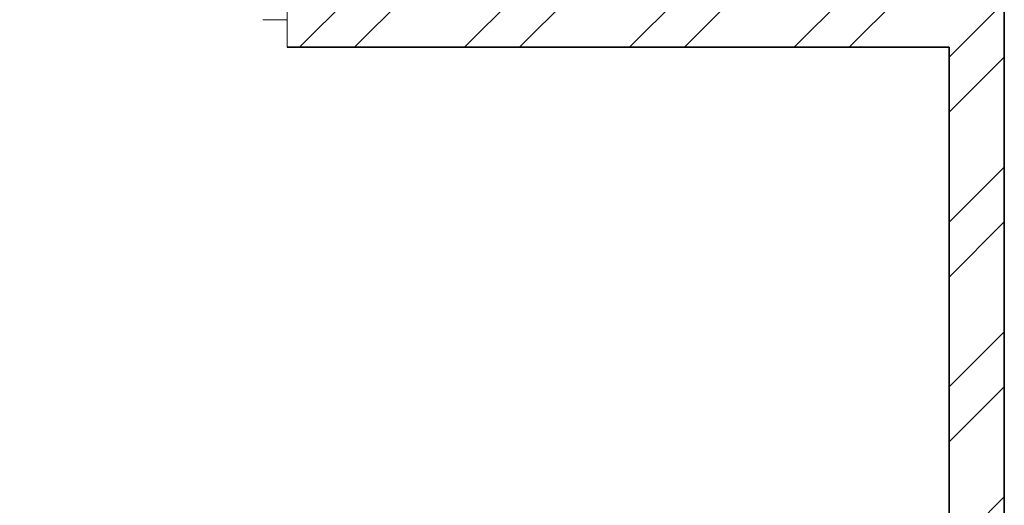
# Model space of a CAD drawing. Units: inches. Extents: x 1962 to 2771, y 1245 to 2660.
# Tile 15 of 114: x 2580 to 2661, y 1609 to 1649. Entities that reach past the tile are written whole.
import ezdxf

# ---------------------------------------------------------------- set-up
doc = ezdxf.new("R2010")
doc.units = ezdxf.units.IN
for name, color, linetype, lineweight in [('A-DOOR', 3, 'Continuous', 18), ('A-WALL', 7, 'Continuous', 35), ('A-WALL-PATT', 252, 'Continuous', 13)]:
    doc.layers.add(name, color=color, linetype=linetype, lineweight=lineweight)

msp = doc.modelspace()

# ---------------------------------------------------------------- hatches: boundary and pattern name
at = {"layer": 'A-WALL-PATT'}
h = msp.add_hatch(dxfattribs=at)
h.set_pattern_fill('ANSI32', color=256)
h.paths.add_polyline_path([(2090.8074, 2467.3437), (2141.6481, 2467.3437), (2141.6481, 2469.5937), (2141.6481, 2471.8437), (2086.3074, 2471.8437), (2086.3074, 2422.5333), (2090.8074, 2422.5333)])
h.paths.add_polyline_path([(2282.7664, 2471.8437), (2204.8982, 2471.8437), (2204.8982, 2467.3437), (2234.8074, 2467.3437), (2234.8074, 2311.3437), (2228.7492, 2311.3437), (2228.7492, 2306.8437), (2234.8074, 2306.8437), (2331.9227, 2306.8437), (2331.9227, 2309.0937), (2331.9227, 2311.3437), (2239.3074, 2311.3437), (2239.3074, 2467.3437), (2282.7664, 2467.3437), (2282.7664, 2469.5937)])
h.paths.add_polyline_path([(2471.4531, 2519.8437), (2552.011, 2519.8437), (2564.3996, 2519.8437), (2564.3996, 2511.1389), (2568.8996, 2511.1389), (2568.8996, 2524.3437), (2466.9531, 2524.3437), (2466.9531, 2471.8437), (2450.0749, 2471.8437), (2446.4672, 2471.8437), (2446.4672, 2467.3437), (2450.0749, 2467.3437), (2475.9988, 2467.3437), (2475.9988, 2469.5937), (2475.9988, 2471.8437), (2471.4531, 2471.8437)])
h.paths.add_polyline_path([(2575.2231, 2469.5937), (2575.2231, 2471.8437), (2568.8996, 2471.8437), (2568.8996, 2487.1389), (2564.3996, 2487.1389), (2564.3996, 2471.8437), (2556.511, 2471.8437), (2499.2904, 2471.8437), (2499.2904, 2467.3437), (2507.8074, 2467.3437), (2507.8074, 2311.3437), (2414.863, 2311.3437), (2414.863, 2306.8437), (2512.3074, 2306.8437), (2517.0114, 2306.8437), (2517.0114, 2309.0937), (2517.0114, 2311.3437), (2512.3074, 2311.3437), (2512.3074, 2467.3437), (2575.2231, 2467.3437)])
h.paths.add_polyline_path([(2660.8074, 2471.8437), (2600.9602, 2471.8437), (2600.9602, 2467.3437), (2656.3074, 2467.3437), (2656.3074, 2432.5704), (2660.8074, 2432.5704)])
h.paths.add_polyline_path([(2660.8074, 2372.5704), (2656.3074, 2372.5704), (2656.3074, 2311.3437), (2600.276, 2311.3437), (2600.276, 2309.0937), (2600.276, 2306.8437), (2656.3074, 2306.8437), (2656.3074, 2296.2593), (2660.8074, 2296.2593)])
h.paths.add_polyline_path([(2572.3074, 2306.8437), (2577.1385, 2306.8437), (2577.1385, 2311.3437), (2551.082, 2311.3437), (2551.082, 2306.8437), (2567.8074, 2306.8437), (2567.8074, 2258.8437), (2540.0574, 2258.8437), (2540.0574, 2256.5937), (2540.0574, 2254.3437), (2567.8074, 2254.3437), (2656.3074, 2254.3437), (2656.3074, 2236.9085), (2660.8074, 2236.9085), (2660.8074, 2272.2593), (2656.3074, 2272.2593), (2656.3074, 2258.8437), (2572.3074, 2258.8437)])
h.paths.add_polyline_path([(2512.3074, 2254.3437), (2518.8716, 2254.3437), (2518.8716, 2256.5937), (2518.8716, 2258.8437), (2507.8074, 2258.8437), (2507.8074, 2177.8437), (2567.8074, 2177.8437), (2567.8074, 2172.9628), (2572.3074, 2172.9628), (2572.3074, 2177.8437), (2656.3074, 2177.8437), (2656.3074, 2166.4846), (2660.8074, 2166.4846), (2660.8074, 2200.9085), (2656.3074, 2200.9085), (2656.3074, 2182.3437), (2512.3074, 2182.3437)])
h.paths.add_polyline_path([(2656.3074, 2129.8437), (2572.3074, 2129.8437), (2572.3074, 2150.3044), (2570.0574, 2150.3044), (2567.8074, 2150.3044), (2567.8074, 2129.8437), (2507.8074, 2129.8437), (2507.8074, 2116.3027), (2510.0574, 2116.3027), (2512.3074, 2116.3027), (2512.3074, 2125.3437), (2567.8074, 2125.3437), (2572.3074, 2125.3437), (2656.3074, 2125.3437)])
h.paths.add_polyline_path([(2090.8074, 2362.5333), (2086.3074, 2362.5333), (2086.3074, 2298.6242), (2090.8074, 2298.6242), (2090.8074, 2306.8437), (2174.8074, 2306.8437), (2174.8074, 2286.4178), (2179.3074, 2286.4178), (2179.3074, 2306.8437), (2192.8641, 2306.8437), (2192.8641, 2309.0937), (2192.8641, 2311.3437), (2090.8074, 2311.3437)])
h.paths.add_polyline_path([(2209.156, 2258.8437), (2179.3074, 2258.8437), (2179.3074, 2263.2236), (2177.0574, 2263.2236), (2174.8074, 2263.2236), (2174.8074, 2258.8437), (2090.8074, 2258.8437), (2090.8074, 2274.6242), (2086.3074, 2274.6242), (2086.3074, 2238.2967), (2088.5574, 2238.2967), (2090.8074, 2238.2967), (2090.8074, 2254.3437), (2209.156, 2254.3437)])
h.paths.add_polyline_path([(2090.8074, 2177.8437), (2234.8074, 2177.8437), (2234.8074, 2173.1428), (2239.3074, 2173.1428), (2239.3074, 2258.8437), (2230.8442, 2258.8437), (2230.8442, 2256.5937), (2230.8442, 2254.3437), (2234.8074, 2254.3437), (2234.8074, 2182.3437), (2090.8074, 2182.3437), (2090.8074, 2202.2967), (2086.3074, 2202.2967), (2086.3074, 2140.0389), (2090.8074, 2140.0389)])
h.paths.add_polyline_path([(2090.8074, 2080.0389), (2086.3074, 2080.0389), (2086.3074, 2033.8437), (2090.8074, 2033.8437)], flags=17)
h.paths.add_polyline_path([(2244.9405, 2033.8437), (2239.3074, 2033.8437), (2239.3074, 2142.0665), (2237.2592, 2142.0665), (2234.8074, 2142.0665), (2234.8074, 2033.8437), (2090.8074, 2033.8437), (2076.5204, 2033.8437), (2072.0204, 2033.8437), (2072.0204, 2000.4493), (2076.5204, 2000.4493), (2076.5204, 2029.3437), (2090.8074, 2029.3437), (2244.9405, 2029.3437), (2244.9405, 2031.5937)])
h.paths.add_polyline_path([(2234.8074, 1933.3437), (2076.5204, 1933.3437), (2076.5204, 1952.4493), (2074.2704, 1952.4493), (2072.0204, 1952.4493), (2072.0204, 1933.3437), (2072.0204, 1928.8437), (2234.8074, 1928.8437)])
h.paths.add_polyline_path([(2090.8074, 1928.8437), (2086.3074, 1928.8437), (2086.3074, 1906.5013), (2090.8074, 1906.5013)])
h.paths.add_polyline_path([(2090.8074, 1846.5013), (2086.3074, 1846.5013), (2086.3074, 1769.9917), (2088.5574, 1769.9917), (2090.8074, 1769.9917), (2090.8074, 1780.3437), (2234.8074, 1780.3437), (2234.8074, 1708.3437), (2230.3764, 1708.3437), (2230.3764, 1703.8437), (2239.3074, 1703.8437), (2239.3074, 1792.6669), (2237.0574, 1792.6669), (2234.8074, 1792.6669), (2234.8074, 1784.8437), (2090.8074, 1784.8437)])
h.paths.add_polyline_path([(2239.3074, 1928.8437), (2244.9405, 1928.8437), (2244.9405, 1931.0937), (2244.9405, 1933.3437), (2234.8074, 1933.3437), (2234.8074, 1928.8437), (2234.8074, 1825.5949), (2239.3074, 1825.5949)])
h.paths.add_polyline_path([(2148.0425, 1649.0937), (2148.0425, 1651.3437), (2090.8074, 1651.3437), (2090.8074, 1646.8437), (2148.0425, 1646.8437)], flags=0)
h.paths.add_polyline_path([(2207.5601, 1708.3437), (2090.8074, 1708.3437), (2090.8074, 1703.8437), (2174.8074, 1703.8437), (2174.8074, 1651.3437), (2170.4457, 1651.3437), (2170.4457, 1646.8437), (2195.9924, 1646.8437), (2195.9924, 1649.0937), (2195.9924, 1651.3437), (2179.3074, 1651.3437), (2179.3074, 1703.8437), (2207.5601, 1703.8437), (2207.5601, 1706.0937)])
h.paths.add_polyline_path([(2090.8074, 1733.9917), (2086.3074, 1733.9917), (2086.3074, 1696.1032), (2088.5574, 1696.1032), (2090.8074, 1696.1032)])
h.paths.add_polyline_path([(2090.8074, 1672.1032), (2086.3074, 1672.1032), (2086.3074, 1600.3335), (2090.8074, 1600.3335)])
h.paths.add_polyline_path([(2090.8074, 1540.3335), (2086.3074, 1540.3335), (2086.3074, 1486.3437), (2139.6766, 1486.3437), (2139.6766, 1490.8437), (2090.8074, 1490.8437)])
h.paths.add_polyline_path([(2302.3876, 1490.8437), (2239.3074, 1490.8437), (2239.3074, 1646.8437), (2335.9994, 1646.8437), (2335.9994, 1651.3437), (2229.884, 1651.3437), (2229.884, 1646.8437), (2234.8074, 1646.8437), (2234.8074, 1490.8437), (2202.7103, 1490.8437), (2202.7103, 1488.5937), (2202.7103, 1486.3437), (2275.0699, 1486.3437), (2275.0699, 1475.772), (2279.5699, 1475.772), (2279.5699, 1486.3437), (2302.3876, 1486.3437)])
h.paths.add_polyline_path([(2279.5699, 1451.772), (2275.0699, 1451.772), (2275.0699, 1438.3437), (2174.8074, 1438.3437), (2174.8074, 1486.3437), (2179.7922, 1486.3437), (2179.7922, 1490.8437), (2163.3585, 1490.8437), (2163.3585, 1488.5937), (2163.3585, 1486.3437), (2170.3074, 1486.3437), (2170.3074, 1433.8437), (2279.5699, 1433.8437)])
h.paths.add_polyline_path([(2427.2363, 1490.8437), (2375.8074, 1490.8437), (2375.8074, 1646.8437), (2381.6401, 1646.8437), (2381.6401, 1651.3437), (2365.887, 1651.3437), (2365.887, 1649.0937), (2365.887, 1646.8437), (2371.3074, 1646.8437), (2371.3074, 1490.8437), (2327.5627, 1490.8437), (2327.5627, 1488.5937), (2327.5627, 1486.3437), (2371.3074, 1486.3437), (2371.3074, 1433.8437), (2375.8074, 1433.8437), (2375.8074, 1486.3437), (2427.2363, 1486.3437)])
h.paths.add_polyline_path([(2512.3074, 1646.8437), (2519.4351, 1646.8437), (2519.4351, 1649.0937), (2519.4351, 1651.3437), (2507.8074, 1651.3437), (2416.0063, 1651.3437), (2416.0063, 1649.0937), (2416.0063, 1646.8437), (2507.8074, 1646.8437), (2507.8074, 1490.8437), (2497.0532, 1490.8437), (2497.0532, 1488.5937), (2497.0532, 1486.3437), (2574.9344, 1486.3437), (2574.9344, 1476.0181), (2579.4344, 1476.0181), (2579.4344, 1486.3437), (2584.4872, 1486.3437), (2584.3074, 1490.8437), (2512.3074, 1490.8437)])
h.paths.add_polyline_path([(2470.5091, 1486.3437), (2473.9767, 1486.3437), (2473.9767, 1490.8437), (2449.6605, 1490.8437), (2449.6605, 1488.5937), (2449.6605, 1486.3437), (2466.0091, 1486.3437), (2466.0091, 1433.8437), (2470.5091, 1433.8437), (2579.4344, 1433.8437), (2579.4344, 1452.0181), (2574.9344, 1452.0181), (2574.9344, 1438.3437), (2554.5091, 1438.3437), (2470.5091, 1438.3437)])
h.paths.add_polyline_path([(2656.3074, 1490.8437), (2611.86, 1490.8437), (2611.86, 1486.3437), (2656.3074, 1486.3437)])
h.paths.add_polyline_path([(2660.8074, 1532.7007), (2658.5574, 1532.7007), (2656.3074, 1532.7007), (2656.3074, 1486.3437), (2660.8074, 1486.3437)])
h.paths.add_polyline_path([(2660.8074, 1664.9663), (2656.3074, 1664.9663), (2656.3074, 1651.3437), (2602.2313, 1651.3437), (2602.2313, 1646.8437), (2656.3074, 1646.8437), (2656.3074, 1592.7007), (2660.8074, 1592.7007)])
h.paths.add_polyline_path([(2660.8074, 1724.5221), (2656.3074, 1724.5221), (2656.3074, 1703.8437), (2542.4725, 1703.8437), (2542.4725, 1699.3437), (2567.8074, 1699.3437), (2567.8074, 1651.3437), (2552.7766, 1651.3437), (2552.7766, 1649.0937), (2552.7766, 1646.8437), (2577.2878, 1646.8437), (2577.2878, 1649.0937), (2577.2878, 1651.3437), (2572.3074, 1651.3437), (2572.3074, 1699.3437), (2656.3074, 1699.3437), (2656.3074, 1688.9663), (2660.8074, 1688.9663)])
h.paths.add_polyline_path([(2660.8074, 1880.6524), (2656.3074, 1880.6524), (2656.3074, 1832.8437), (2512.3074, 1832.8437), (2512.3074, 1837.8959), (2507.8074, 1837.8959), (2507.8074, 1828.3437), (2567.8074, 1828.3437), (2567.8074, 1804.3437), (2572.3074, 1804.3437), (2572.3074, 1828.3437), (2656.3074, 1828.3437), (2656.3074, 1818.6778), (2660.8074, 1818.6778)])
h.paths.add_polyline_path([(2660.8074, 1794.6778), (2656.3074, 1794.6778), (2656.3074, 1780.3437), (2572.3074, 1780.3437), (2572.3074, 1783.0303), (2570.0574, 1783.0303), (2567.8074, 1783.0303), (2567.8074, 1780.3437), (2507.8074, 1780.3437), (2507.8074, 1699.3437), (2517.8858, 1699.3437), (2517.8858, 1701.5937), (2517.8858, 1703.8437), (2512.3074, 1703.8437), (2512.3074, 1775.8437), (2656.3074, 1775.8437), (2656.3074, 1760.5221), (2660.8074, 1760.5221)])
h.paths.add_polyline_path([(2660.8074, 1981.3437), (2660.8074, 2020.2808), (2658.5574, 2020.2808), (2656.3074, 2020.2808), (2656.3074, 1981.3437), (2512.3074, 1981.3437), (2512.3074, 2086.6996), (2507.8074, 2086.6996), (2507.8074, 1981.3437), (2375.8074, 1981.3437), (2375.8074, 1986.8505), (2373.5574, 1986.8505), (2371.3074, 1986.8505), (2371.3074, 1973.2607), (2375.8074, 1973.2607), (2375.8074, 1976.8437), (2507.8074, 1976.8437), (2507.8074, 1865.4281), (2510.0574, 1865.4281), (2512.3074, 1865.4281), (2512.3074, 1976.8437), (2660.8074, 1976.8437)])
h.paths.add_polyline_path([(2375.8074, 1940.297), (2373.5574, 1940.297), (2371.3074, 1940.297), (2371.3074, 1933.3437), (2278.4434, 1933.3437), (2278.4434, 1928.8437), (2371.3074, 1928.8437), (2371.3074, 1651.3437), (2375.8074, 1651.3437)])
h.paths.add_polyline_path([(2660.8074, 1976.8437), (2656.3074, 1976.8437), (2656.3074, 1940.6524), (2660.8074, 1940.6524)], flags=17)
h.paths.add_polyline_path([(2660.8074, 2142.4846), (2656.3074, 2142.4846), (2656.3074, 2080.2808), (2660.8074, 2080.2808)])
h.paths.add_polyline_path([(2381.4189, 2311.3437), (2375.8074, 2311.3437), (2375.8074, 2467.3437), (2424.7242, 2467.3437), (2424.7242, 2469.5937), (2424.7242, 2471.8437), (2375.8074, 2471.8437), (2375.8074, 2524.3437), (2371.3074, 2524.3437), (2371.3074, 2471.8437), (2307.2097, 2471.8437), (2307.2097, 2467.3437), (2371.3074, 2467.3437), (2371.3074, 2311.3437), (2366.8901, 2311.3437), (2366.8901, 2306.8437), (2371.3074, 2306.8437), (2371.3074, 2033.8437), (2279.6589, 2033.8437), (2279.6589, 2029.3437), (2371.3074, 2029.3437), (2371.3074, 2014.2598), (2375.8074, 2014.2598), (2375.8074, 2306.8437), (2381.4189, 2306.8437)])
h.paths.add_polyline_path([(2263.3074, 2524.3437), (2170.3074, 2524.3437), (2170.3074, 2519.8437), (2170.3074, 2471.8437), (2165.0312, 2471.8437), (2165.0312, 2467.3437), (2179.6721, 2467.3437), (2179.6721, 2469.5161), (2179.6721, 2471.8437), (2174.8074, 2471.8437), (2174.8074, 2519.8437), (2258.8074, 2519.8437), (2258.8074, 2511.6436), (2263.3074, 2511.6436)])
h.paths.add_polyline_path([(2245.0232, 1361.4123), (2492.9468, 1361.4123), (2492.9468, 1398.505), (2245.0232, 1398.505)], flags=9)
h.paths.add_polyline_path([(2388.1434, 2086.6936), (2425.0704, 2086.6936), (2425.0704, 2105.3509), (2388.1434, 2105.3509)], flags=9)
h.paths.add_polyline_path([(2404.922, 2242.6744), (2445.7337, 2242.6744), (2445.7337, 2261.3318), (2404.922, 2261.3318)], flags=9)
h.paths.add_polyline_path([(2269.4107, 2156.7935), (2306.3378, 2156.7935), (2306.3378, 2175.4508), (2269.4107, 2175.4508)], flags=9)
h.paths.add_polyline_path([(2269.3277, 2233.4343), (2306.2547, 2233.4343), (2306.2547, 2252.0917), (2269.3277, 2252.0917)], flags=9)
h.paths.add_polyline_path([(2431.6052, 2320.6922), (2470.4456, 2320.6922), (2470.4456, 2339.3495), (2431.6052, 2339.3495)], flags=25)
h.paths.add_polyline_path([(2249.6902, 2315.7608), (2288.5306, 2315.7608), (2288.5306, 2334.4182), (2249.6902, 2334.4182)], flags=25)
h.paths.add_polyline_path([(2096.9301, 2314.3181), (2135.7704, 2314.3181), (2135.7704, 2332.9755), (2096.9301, 2332.9755)], flags=25)
h.paths.add_polyline_path([(2134.3475, 2285.7089), (2161.4655, 2285.7089), (2161.4655, 2304.3662), (2134.3475, 2304.3662)], flags=9)
h.paths.add_polyline_path([(2126.5155, 2209.4076), (2159.9227, 2209.4076), (2159.9227, 2228.065), (2126.5155, 2228.065)], flags=25)
h.paths.add_polyline_path([(2110.5753, 2141.5299), (2149.4157, 2141.5299), (2149.4157, 2160.1872), (2110.5753, 2160.1872)], flags=25)
h.paths.add_polyline_path([(2249.8618, 1968.3317), (2286.3966, 1968.3317), (2286.3966, 1986.989), (2249.8618, 1986.989)], flags=9)
h.paths.add_polyline_path([(2395.9507, 1777.0051), (2436.7624, 1777.0051), (2436.7624, 1795.6625), (2395.9507, 1795.6625)], flags=9)
h.paths.add_polyline_path([(2398.5259, 1888.5651), (2435.0062, 1888.5651), (2435.0062, 1907.2224), (2398.5259, 1907.2224)], flags=25)
h.paths.add_polyline_path([(2259.3506, 1728.3559), (2296.2776, 1728.3559), (2296.2776, 1747.0132), (2259.3506, 1747.0132)], flags=9)
h.paths.add_polyline_path([(2271.3698, 1845.268), (2308.2968, 1845.268), (2308.2968, 1863.9253), (2271.3698, 1863.9253)], flags=9)
h.paths.add_polyline_path([(2120.9355, 1786.3027), (2159.7759, 1786.3027), (2159.7759, 1804.9601), (2120.9355, 1804.9601)], flags=25)
h.paths.add_polyline_path([(2121.3164, 1732.1043), (2154.7236, 1732.1043), (2154.7236, 1750.7616), (2121.3164, 1750.7616)], flags=25)
h.paths.add_polyline_path([(2118.3706, 1678.8997), (2147.5282, 1678.8997), (2147.5282, 1697.557), (2118.3706, 1697.557)], flags=25)
h.paths.add_polyline_path([(2385.9227, 1493.557), (2424.763, 1493.557), (2424.763, 1512.2143), (2385.9227, 1512.2143)], flags=25)
h.paths.add_polyline_path([(2248.7058, 1500.0256), (2287.5462, 1500.0256), (2287.5462, 1518.6829), (2248.7058, 1518.6829)], flags=25)
h.paths.add_polyline_path([(2104.1669, 1617.3771), (2143.0073, 1617.3771), (2143.0073, 1636.0344), (2104.1669, 1636.0344)], flags=9)
h.paths.add_polyline_path([(2096.0714, 1447.8824), (2137.3845, 1447.8824), (2137.3845, 1458.1859), (2096.0714, 1458.1859)], flags=9)
h.paths.add_polyline_path([(2180.6114, 1440.325), (2209.7689, 1440.325), (2209.7689, 1458.9823), (2180.6114, 1458.9823)], flags=25)
h.paths.add_polyline_path([(2316.1698, 1447.9637), (2357.4829, 1447.9637), (2357.4829, 1458.2673), (2316.1698, 1458.2673)], flags=9)
h.paths.add_polyline_path([(2397.6187, 1447.9637), (2438.9318, 1447.9637), (2438.9318, 1458.2673), (2397.6187, 1458.2673)], flags=9)
h.paths.add_polyline_path([(2473.0778, 1439.5953), (2502.2354, 1439.5953), (2502.2354, 1458.2527), (2473.0778, 1458.2527)], flags=25)
h.paths.add_polyline_path([(2589.7027, 1447.8819), (2631.0158, 1447.8819), (2631.0158, 1458.1855), (2589.7027, 1458.1855)], flags=9)
h.paths.add_polyline_path([(2522.4009, 1497.5285), (2561.2413, 1497.5285), (2561.2413, 1516.1859), (2522.4009, 1516.1859)], flags=25)
h.paths.add_polyline_path([(2579.6565, 1671.3482), (2608.8141, 1671.3482), (2608.8141, 1690.0056), (2579.6565, 1690.0056)], flags=25)
h.paths.add_polyline_path([(2544.7038, 1725.5064), (2578.1111, 1725.5064), (2578.1111, 1744.1637), (2544.7038, 1744.1637)], flags=25)
h.paths.add_polyline_path([(2578.1191, 1807.472), (2607.2766, 1807.472), (2607.2766, 1826.1293), (2578.1191, 1826.1293)], flags=25)
h.paths.add_polyline_path([(2595.0614, 1835.1839), (2633.9018, 1835.1839), (2633.9018, 1853.8413), (2595.0614, 1853.8413)], flags=25)
h.paths.add_polyline_path([(2567.0097, 2097.7035), (2605.8501, 2097.7035), (2605.8501, 2116.3609), (2567.0097, 2116.3609)], flags=9)
h.paths.add_polyline_path([(2586.644, 2134.6454), (2615.8015, 2134.6454), (2615.8015, 2153.3027), (2586.644, 2153.3027)], flags=9)
h.paths.add_polyline_path([(2544.6185, 2212.6783), (2578.0258, 2212.6783), (2578.0258, 2231.3356), (2544.6185, 2231.3356)], flags=25)
h.paths.add_polyline_path([(2577.0273, 2256.9023), (2606.1849, 2256.9023), (2606.1849, 2275.5597), (2577.0273, 2275.5597)], flags=24)
h.paths.add_polyline_path([(2605.2683, 2315.2821), (2644.1087, 2315.2821), (2644.1087, 2333.9395), (2605.2683, 2333.9395)], flags=25)
h.paths.add_polyline_path([(2583.1244, 2496.1815), (2624.4375, 2496.1815), (2624.4375, 2506.4851), (2583.1244, 2506.4851)], flags=9)
h.paths.add_polyline_path([(2474.761, 2497.0823), (2503.9185, 2497.0823), (2503.9185, 2515.7397), (2474.761, 2515.7397)], flags=25)
h.paths.add_polyline_path([(2387.5787, 2494.2563), (2428.902, 2494.2563), (2428.902, 2504.5598), (2387.5787, 2504.5598)], flags=9)
h.paths.add_polyline_path([(2300.1657, 2500.1564), (2341.4788, 2500.1564), (2341.4788, 2510.46), (2300.1657, 2510.46)], flags=25)
h.paths.add_polyline_path([(2176.8589, 2497.5843), (2206.0165, 2497.5843), (2206.0165, 2516.2416), (2176.8589, 2516.2416)], flags=25)
h.paths.add_polyline_path([(2097.4668, 2494.9762), (2138.7799, 2494.9762), (2138.7799, 2505.2798), (2097.4668, 2505.2798)], flags=9)

# ---------------------------------------------------------------- linework, layer by layer
at = {"layer": 'A-DOOR'}
for p, q in [((2602.2313, 1651.3437), (2602.2313, 1646.8437)), ((2602.2313, 1649.0937), (2600.2313, 1649.0937)), ((2602.2313, 1646.8437), (2602.2313, 1649.0937))]:
    msp.add_line(p, q, dxfattribs=at)
at = {"layer": 'A-WALL'}
for p, q in [((2660.8074, 1976.8437), (2660.8074, 1486.3437)), ((2656.3074, 1646.8437), (2602.2313, 1646.8437)), ((2656.3074, 1646.8437), (2656.3074, 1486.3437))]:
    msp.add_line(p, q, dxfattribs=at)

doc.saveas('drawing.dxf')
